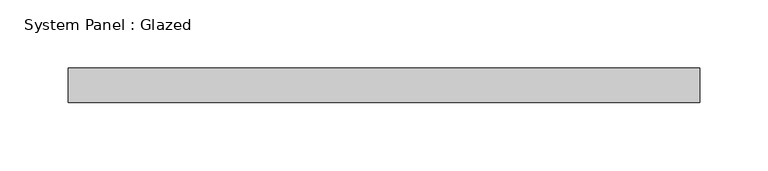
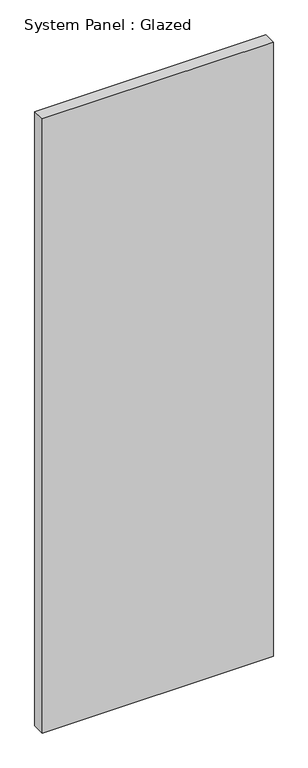
"""IFC4 building model written with IfcOpenShell, lengths in millimetres: plate geometry, System Panel : Glazed."""

from ifc_helpers import new_model, si_unit, origin, origin_with_axes, place, context, project, spatial, polyline, outline, extrude, source, transform, mapped, element, save


def system_panel_glazed_bdc4a67b(model_context):
    return source(origin(), model_context, "Body", "SweptSolid", [
        extrude(outline(polyline([(231.775, 19.05), (-231.775, 19.05), (-231.775, 44.45), (231.775, 44.45), (231.775, 19.05)])), origin_with_axes(), (0.0, 0.0, 1.0), 1301.2525568),
    ])


if __name__ == "__main__":
    model = new_model("IFC4")
    model_context = context("Model", 3, world=origin())
    ifc_project = project(units=[si_unit("LENGTHUNIT", "METRE", prefix="MILLI")], contexts=[model_context])
    site = spatial("IfcSite", under=ifc_project)
    building = spatial("IfcBuilding", under=site)
    placement = place(None, origin())
    system_panel_glazed_shape = system_panel_glazed_bdc4a67b(model_context)
    element("IfcPlate", 1, ObjectType="System Panel : Glazed", at=placement, inside=building, context=model_context, shape_type="MappedRepresentation", body=[
        mapped(system_panel_glazed_shape, transform((0.0, 0.0, 0.0), x_axis=(1.0, 0.0, 0.0), y_axis=(0.0, 1.0, 0.0), z_axis=(0.0, 0.0, 1.0))),
    ])
    save(model, "model.ifc")

# Revit data of these elements
# Type "System Panel : Glazed"
#   Construction Type Id = "GSP4R"
#   Analytic Construction = "1/8 in Pilkington single glazing"
#   Visual Light Transmittance = 0.9
#   Solar Heat Gain Coefficient = 0.86
#   Heat Transfer Coefficient (U) = 1.18115 BTU/(h·ft²·°F)
#   Define Thermal Properties by = 1
# Element 1 (IfcPlate, "System Panel : Glazed")
#   Materials on its faces: "Glass"
# Materials
#   "Glass": class "Glass", colour RGB 0 128 192, transparency 0.75, Description = "Soda Lime Glass", Cost = 0
